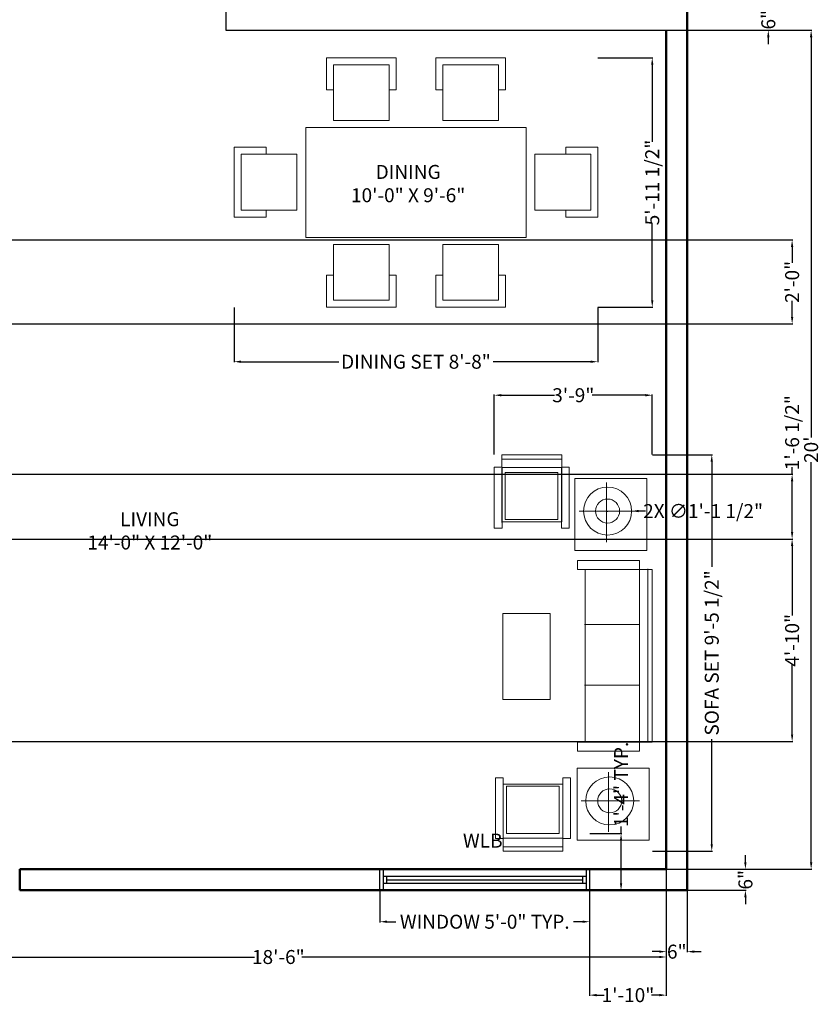
# Model space of a CAD drawing. Units: inches. Extents: x 2663 to 3147, y 140 to 736.
# Tile 3 of 6: x 2905 to 3134, y 144 to 425. Entities that reach past the tile are written whole.
import ezdxf

# ---------------------------------------------------------------- set-up
doc = ezdxf.new("R2010")
doc.units = ezdxf.units.IN
doc.header["$MEASUREMENT"] = 0
for name, color, linetype, lineweight in [('A-ANNO-DIMS', 2, 'Continuous', 18), ('A-AREA-IDEN', 3, 'Continuous', 25), ('A-FLOR-STRS', 1, 'Continuous', 25), ('A-FURN', 8, 'Continuous', 18), ('A-GLAZ', 4, 'Continuous', 25), ('A-WALL', 7, 'Continuous', 50)]:
    doc.layers.add(name, color=color, linetype=linetype, lineweight=lineweight)
doc.styles.get("Standard").update_dxf_attribs({"font": 'arial.ttf'})
doc.dimstyles.get("Standard").update_dxf_attribs({"dimtxt": 4, "dimasz": 2, "dimexe": 0.18, "dimexo": 0.0625, "dimgap": 0.09, "dimtad": 0, "dimdec": 0, "dimzin": 0, "dimdsep": 46, "dimlunit": 4, "dimtxsty": 'Standard', "dimcen": 0.09, "dimadec": 0, "dimazin": 0, "dimtfac": 1, "dimtdec": 0, "dimtofl": 0, "dimtmove": 0, "dimatfit": 3, "dimfxl": 1, "dimtolj": 1, "dimtzin": 0, "dimarcsym": 0})

# ---------------------------------------------------------------- blocks, each defined once
blk = doc.blocks.new('EDFRTYUI')
for p, q in [((3325.9, 253.54), (3325.9, 259.54)), ((3325.9, 259.54), (3385.9, 259.54)), ((3326.9, 253.54), (3326.9, 259.54)), ((3384.9, 259.54), (3384.9, 253.54)), ((3385.9, 259.54), (3385.9, 253.54)), ((3326.9, 257.54), (3384.9, 257.54)), ((3327.9, 255.54), (3327.9, 257.54)), ((3327.9, 256.54), (3383.9, 256.54)), ((3383.9, 257.54), (3383.9, 255.54)), ((3385.9, 253.54), (3325.9, 253.54)), ((3326.9, 255.54), (3384.9, 255.54))]:
    blk.add_line(p, q)
at = {"insert": (3337.87, 269.72), "char_height": 4, "attachment_point": 1}
blk.add_mtext_dynamic_manual_height_columns('\\pxqc;WLB', width=34.9199, gutter_width=20, heights=[0], dxfattribs=at)
blk = doc.blocks.new('A$C30E17696')
for p, q in [((0.6703, 1.8113), (1.177, 1.8113)), ((0.6703, 1.8113), (0.6703, 1.5785)), ((1.177, 1.8113), (1.177, 1.5785)), ((1.9712, 1.8113), (1.4645, 1.8113)), ((1.4645, 1.8113), (1.4645, 1.5785)), ((1.9712, 1.8113), (1.9712, 1.5785)), ((0.7209, 1.7606), (0.7209, 1.3552)), ((0.7209, 1.7606), (1.1263, 1.7606)), ((1.1263, 1.7606), (1.1263, 1.3552)), ((1.5151, 1.7606), (1.5151, 1.3552)), ((1.9205, 1.7606), (1.5151, 1.7606)), ((1.9205, 1.7606), (1.9205, 1.3552)), ((0.6703, 1.5785), (0.7209, 1.5785)), ((1.1263, 1.5785), (1.177, 1.5785)), ((1.5151, 1.5785), (1.4645, 1.5785)), ((1.9712, 1.5785), (1.9205, 1.5785)), ((0.5207, 1.3056), (0.5207, 0.5056)), ((2.1207, 1.3056), (0.5207, 1.3056)), ((0.7209, 1.3552), (1.1263, 1.3552)), ((1.9205, 1.3552), (1.5151, 1.3552)), ((2.1207, 0.5056), (2.1207, 1.3056)), ((0, 0.6545), (0, 1.1613)), ((0, 1.1613), (0.2327, 1.1613)), ((0.2327, 1.1106), (0.2327, 1.1613)), ((2.6414, 1.1613), (2.4087, 1.1613)), ((2.4087, 1.1106), (2.4087, 1.1613)), ((2.6414, 0.6545), (2.6414, 1.1613)), ((0.0507, 0.7052), (0.0507, 1.1106)), ((0.0507, 1.1106), (0.456, 1.1106)), ((0.456, 0.7052), (0.456, 1.1106)), ((2.1854, 0.7052), (2.1854, 1.1106)), ((2.5907, 1.1106), (2.1854, 1.1106)), ((2.5907, 0.7052), (2.5907, 1.1106)), ((0, 0.6545), (0.2327, 0.6545)), ((0.0507, 0.7052), (0.456, 0.7052)), ((0.2327, 0.6545), (0.2327, 0.7052)), ((2.5907, 0.7052), (2.1854, 0.7052)), ((2.4087, 0.6545), (2.4087, 0.7052)), ((2.6414, 0.6545), (2.4087, 0.6545)), ((0.5207, 0.5056), (2.1207, 0.5056)), ((0.7209, 0.456), (1.1263, 0.456)), ((0.7209, 0.0507), (0.7209, 0.456)), ((1.1263, 0.0507), (1.1263, 0.456)), ((1.5151, 0.0507), (1.5151, 0.456)), ((1.9205, 0.456), (1.5151, 0.456)), ((1.9205, 0.0507), (1.9205, 0.456)), ((0.6703, 0), (0.6703, 0.2327)), ((0.6703, 0.2327), (0.7209, 0.2327)), ((1.1263, 0.2327), (1.177, 0.2327)), ((1.177, 0), (1.177, 0.2327)), ((1.4645, 0), (1.4645, 0.2327)), ((1.5151, 0.2327), (1.4645, 0.2327)), ((1.9712, 0.2327), (1.9205, 0.2327)), ((1.9712, 0), (1.9712, 0.2327)), ((0.7209, 0.0507), (1.1263, 0.0507)), ((1.9205, 0.0507), (1.5151, 0.0507)), ((0.6703, 0), (1.177, 0)), ((1.9712, 0), (1.4645, 0))]:
    blk.add_line(p, q)
blk = doc.blocks.new('A$C482A143B')
for p, q in [((952.8, 1281.2), (2397.2, 1281.2)), ((469.8, 1193.5), (469.8, 706.9)), ((952.8, 1210.8), (2397.2, 1210.8)), ((1416.2, 1204.9), (1416.2, 753.5)), ((1920.6, 1204.9), (1920.6, 753.5)), ((2886.7, 1211), (2886.7, 724.4)), ((231.4, 934.7), (729, 934.7)), ((2648.3, 952.2), (3145.8, 952.2)), ((36.9, 62), (36.9, 562)), ((107.2, 62), (107.2, 562)), ((3198.7, 72.9), (3198.7, 573)), ((3269.1, 72.9), (3269.1, 573)), ((107.2, 62), (0, 62)), ((113.1, 62), (564.6, 62)), ((3192.9, 72.9), (2741.4, 72.9)), ((3198.7, 72.9), (3305.9, 72.9))]:
    blk.add_line(p, q)
for points in [[(957.2, 758), (957.2, 1318), (2397.2, 1318), (2397.2, 758)], [(797.5, 672.9), (197.5, 672.9), (197.5, 1272.9), (797.5, 1272.9)], [(3214.3, 690.4), (2614.3, 690.4), (2614.3, 1290.4), (3214.3, 1290.4)], [(883, 694), (883, 1210.8), (957.2, 1210.8), (957.2, 694)], [(2471.3, 694), (2471.3, 1210.8), (2397.2, 1210.8), (2397.2, 694)], [(611.7, 559.6), (105.3, 559.6), (105.3, 624), (611.7, 624)], [(2694.3, 570.6), (3200.7, 570.6), (3200.7, 634.9), (2694.3, 634.9)], [(541.1, 91.3), (148.3, 91.3), (148.3, 531.2), (541.1, 531.2)], [(2764.8, 102.3), (3157.7, 102.3), (3157.7, 542.2), (2764.8, 542.2)], [(1325.3, 466.6), (2040.7, 466.6), (2040.7, 72.4), (1325.3, 72.4)], [(611.7, 64.4), (105.3, 64.4), (105.3, 0), (611.7, 0)], [(2694.3, 75.4), (3200.7, 75.4), (3200.7, 11), (2694.3, 11)]]:
    blk.add_lwpolyline(points, close=True)
for points in [[(0, 62), (0, 562), (560, 562), (560, 62)], [(3305.9, 72.9), (3305.9, 573), (2745.9, 573), (2745.9, 72.9)]]:
    blk.add_lwpolyline(points)
for centre, radius in [((2886.7, 962.5), 200), ((469.8, 945), 200), ((469.8, 945), 100), ((2886.7, 962.5), 100)]:
    blk.add_circle(centre, radius)
at = {"width": 0.8, "flags": 9}
for tag in ['XSIZE', 'YSIZE']:
    blk.add_attdef(tag, (1677.2, 758), '', height=0.4, dxfattribs=at)
for tag in ['XSIZE', 'YSIZE']:
    blk.add_attdef(tag, (541.1, 311.2), '', height=0.4, rotation=90, dxfattribs=at)
at = {"text_generation_flag": 2, "width": 0.8, "flags": 9}
for tag in ['YSIZE', 'XSIZE']:
    blk.add_attdef(tag, (2764.8, 322.2), '', height=0.4, rotation=270, dxfattribs=at)
blk = doc.blocks.new('*D25')
at = {"layer": 'A-ANNO-DIMS', "color": 0, "lineweight": -2, "transparency": 16777216}
for p, q in [((3119.35, 430.32), (3119.35, 432.32)), ((3096.22, 428.32), (3119.53, 428.32)), ((3096.22, 422.32), (3119.53, 422.32)), ((3119.35, 420.32), (3119.35, 418.32))]:
    blk.add_line(p, q, dxfattribs=at)
at = {"layer": 'A-ANNO-DIMS', "color": 0, "transparency": 16777216}
for points in [[(3119.01, 430.32), (3119.68, 430.32), (3119.35, 428.32)], [(3119.01, 420.32), (3119.68, 420.32), (3119.35, 422.32)]]:
    blk.add_solid(points, dxfattribs=at)
at = {"layer": 'Defpoints', "color": 0, "transparency": 16777216}
for p in [(3096.16, 428.32), (3096.16, 422.32), (3119.35, 422.32)]:
    blk.add_point(p, dxfattribs=at)
at = {"layer": 'A-ANNO-DIMS', "color": 0, "transparency": 16777216, "insert": (3119.35, 425.32), "char_height": 4, "attachment_point": 5, "rotation": 90}
blk.add_mtext('\\A1;6"', dxfattribs=at)
blk = doc.blocks.new('*D26')
at = {"layer": 'A-ANNO-DIMS', "color": 0, "lineweight": -2, "transparency": 16777216}
for p, q in [((3090.22, 422.32), (3131.78, 422.32)), ((3131.6, 420.32), (3131.6, 305.84)), ((3131.6, 184.32), (3131.6, 298.81)), ((3090.22, 182.32), (3131.78, 182.32))]:
    blk.add_line(p, q, dxfattribs=at)
at = {"layer": 'A-ANNO-DIMS', "color": 0, "transparency": 16777216}
for points in [[(3131.27, 420.32), (3131.94, 420.32), (3131.6, 422.32)], [(3131.27, 184.32), (3131.94, 184.32), (3131.6, 182.32)]]:
    blk.add_solid(points, dxfattribs=at)
at = {"layer": 'Defpoints', "color": 0, "transparency": 16777216}
for p in [(3090.16, 422.32), (3090.16, 182.32), (3131.6, 182.32)]:
    blk.add_point(p, dxfattribs=at)
at = {"layer": 'A-ANNO-DIMS', "color": 0, "transparency": 16777216, "insert": (3131.6, 302.32), "char_height": 4, "attachment_point": 5, "rotation": 90}
blk.add_mtext("\\A1;20'", dxfattribs=at)
blk = doc.blocks.new('*D27')
at = {"layer": 'A-ANNO-DIMS', "color": 0, "lineweight": -2, "transparency": 16777216}
for p, q in [((2868.16, 182.26), (2868.16, 157.05)), ((3090.16, 182.26), (3090.16, 157.05)), ((2870.16, 157.23), (2972.39, 157.23)), ((3088.16, 157.23), (2985.93, 157.23))]:
    blk.add_line(p, q, dxfattribs=at)
at = {"layer": 'A-ANNO-DIMS', "color": 0, "transparency": 16777216}
for points in [[(2870.16, 157.56), (2870.16, 156.89), (2868.16, 157.23)], [(3088.16, 157.56), (3088.16, 156.89), (3090.16, 157.23)]]:
    blk.add_solid(points, dxfattribs=at)
at = {"layer": 'Defpoints', "color": 0, "transparency": 16777216}
for p in [(2868.16, 182.32), (3090.16, 182.32), (2868.16, 157.23)]:
    blk.add_point(p, dxfattribs=at)
at = {"layer": 'A-ANNO-DIMS', "color": 0, "transparency": 16777216, "insert": (2979.16, 157.23), "char_height": 4, "attachment_point": 5}
blk.add_mtext('\\A1;18\'-6"', dxfattribs=at)
blk = doc.blocks.new('*D28')
at = {"layer": 'A-ANNO-DIMS', "color": 0, "lineweight": -2, "transparency": 16777216}
for p, q in [((3090.16, 182.26), (3090.16, 158.58)), ((3096.16, 176.26), (3096.16, 158.58)), ((3088.16, 158.76), (3086.16, 158.76)), ((3098.16, 158.76), (3100.16, 158.76))]:
    blk.add_line(p, q, dxfattribs=at)
at = {"layer": 'A-ANNO-DIMS', "color": 0, "transparency": 16777216}
for points in [[(3088.16, 159.1), (3088.16, 158.43), (3090.16, 158.76)], [(3098.16, 159.1), (3098.16, 158.43), (3096.16, 158.76)]]:
    blk.add_solid(points, dxfattribs=at)
at = {"layer": 'Defpoints', "color": 0, "transparency": 16777216}
for p in [(3090.16, 182.32), (3096.16, 176.32), (3090.16, 158.76)]:
    blk.add_point(p, dxfattribs=at)
at = {"layer": 'A-ANNO-DIMS', "color": 0, "transparency": 16777216, "insert": (3093.16, 158.76), "char_height": 4, "attachment_point": 5}
blk.add_mtext('\\A1;6"', dxfattribs=at)
blk = doc.blocks.new('*D29')
at = {"layer": 'A-ANNO-DIMS', "color": 0, "lineweight": -2, "transparency": 16777216}
for p, q in [((3112.8, 184.32), (3112.8, 186.32)), ((3090.22, 182.32), (3112.98, 182.32)), ((3096.22, 176.32), (3112.98, 176.32)), ((3112.8, 174.32), (3112.8, 172.32))]:
    blk.add_line(p, q, dxfattribs=at)
at = {"layer": 'A-ANNO-DIMS', "color": 0, "transparency": 16777216}
for points in [[(3112.46, 184.32), (3113.13, 184.32), (3112.8, 182.32)], [(3112.46, 174.32), (3113.13, 174.32), (3112.8, 176.32)]]:
    blk.add_solid(points, dxfattribs=at)
at = {"layer": 'Defpoints', "color": 0, "transparency": 16777216}
for p in [(3090.16, 182.32), (3112.8, 182.32), (3096.16, 176.32)]:
    blk.add_point(p, dxfattribs=at)
at = {"layer": 'A-ANNO-DIMS', "color": 0, "transparency": 16777216, "insert": (3112.8, 179.32), "char_height": 4, "attachment_point": 5, "rotation": 90}
blk.add_mtext('\\A1;6"', dxfattribs=at)
blk = doc.blocks.new('*D41')
at = {"layer": 'A-ANNO-DIMS', "color": 0, "lineweight": -2, "transparency": 16777216}
for p, q in [((3008.22, 176.26), (3008.22, 167.14)), ((3068.22, 176.26), (3068.22, 167.14)), ((3010.22, 167.32), (3012.82, 167.32)), ((3066.22, 167.32), (3063.62, 167.32))]:
    blk.add_line(p, q, dxfattribs=at)
at = {"layer": 'A-ANNO-DIMS', "color": 0, "transparency": 16777216}
for points in [[(3010.22, 167.66), (3010.22, 166.99), (3008.22, 167.32)], [(3066.22, 167.66), (3066.22, 166.99), (3068.22, 167.32)]]:
    blk.add_solid(points, dxfattribs=at)
at = {"layer": 'Defpoints', "color": 0, "transparency": 16777216}
for p in [(3008.22, 176.32), (3068.22, 176.32), (3068.22, 167.32)]:
    blk.add_point(p, dxfattribs=at)
at = {"layer": 'A-ANNO-DIMS', "color": 0, "transparency": 16777216, "insert": (3038.22, 167.32), "char_height": 4, "attachment_point": 5}
blk.add_mtext('\\A1;WINDOW 5\'-0" TYP.', dxfattribs=at)
blk = doc.blocks.new('*D42')
at = {"layer": 'A-ANNO-DIMS', "color": 0, "lineweight": -2, "transparency": 16777216}
for p, q in [((3077.22, 192.51), (3077.22, 194.51)), ((3068.28, 192.51), (3077.4, 192.51)), ((3077.22, 178.32), (3077.22, 190.51)), ((3068.28, 176.32), (3077.4, 176.32))]:
    blk.add_line(p, q, dxfattribs=at)
at = {"layer": 'A-ANNO-DIMS', "color": 0, "transparency": 16777216}
for points in [[(3076.89, 190.51), (3077.55, 190.51), (3077.22, 192.51)], [(3076.89, 178.32), (3077.55, 178.32), (3077.22, 176.32)]]:
    blk.add_solid(points, dxfattribs=at)
at = {"layer": 'Defpoints', "color": 0, "transparency": 16777216}
for p in [(3068.22, 192.51), (3077.22, 192.51), (3068.22, 176.32)]:
    blk.add_point(p, dxfattribs=at)
at = {"layer": 'A-ANNO-DIMS', "color": 0, "transparency": 16777216, "insert": (3077.22, 206.6), "char_height": 4, "attachment_point": 5, "rotation": 90}
blk.add_mtext('\\A1;1\'-4" TYP.', dxfattribs=at)
blk = doc.blocks.new('*D57')
at = {"layer": 'A-ANNO-DIMS', "color": 0, "lineweight": -2, "transparency": 16777216}
for p, q in [((2966.52, 343.04), (2966.52, 327.32)), ((3070.54, 343.04), (3070.54, 327.32)), ((2968.52, 327.5), (2996.46, 327.5)), ((3068.54, 327.5), (3040.6, 327.5))]:
    blk.add_line(p, q, dxfattribs=at)
at = {"layer": 'A-ANNO-DIMS', "color": 0, "transparency": 16777216}
for points in [[(2968.52, 327.83), (2968.52, 327.16), (2966.52, 327.5)], [(3068.54, 327.83), (3068.54, 327.16), (3070.54, 327.5)]]:
    blk.add_solid(points, dxfattribs=at)
at = {"layer": 'Defpoints', "color": 0, "transparency": 16777216}
for p in [(2966.52, 343.1), (3070.54, 343.1), (3070.54, 327.5)]:
    blk.add_point(p, dxfattribs=at)
at = {"layer": 'A-ANNO-DIMS', "color": 0, "transparency": 16777216, "insert": (3018.53, 327.5), "char_height": 4, "attachment_point": 5}
blk.add_mtext('\\A1;DINING SET 8\'-8"', dxfattribs=at)
blk = doc.blocks.new('*D58')
at = {"layer": 'A-ANNO-DIMS', "color": 0, "lineweight": -2, "transparency": 16777216}
for p, q in [((3070.6, 414.42), (3086.32, 414.42)), ((3086.14, 412.42), (3086.14, 390.38)), ((3086.14, 345.1), (3086.14, 367.14)), ((3070.6, 343.1), (3086.32, 343.1))]:
    blk.add_line(p, q, dxfattribs=at)
at = {"layer": 'A-ANNO-DIMS', "color": 0, "transparency": 16777216}
for points in [[(3085.81, 412.42), (3086.47, 412.42), (3086.14, 414.42)], [(3085.81, 345.1), (3086.47, 345.1), (3086.14, 343.1)]]:
    blk.add_solid(points, dxfattribs=at)
at = {"layer": 'Defpoints', "color": 0, "transparency": 16777216}
for p in [(3070.54, 414.42), (3086.14, 414.42), (3070.54, 343.1)]:
    blk.add_point(p, dxfattribs=at)
at = {"layer": 'A-ANNO-DIMS', "color": 0, "transparency": 16777216, "insert": (3086.14, 378.76), "char_height": 4, "attachment_point": 5, "rotation": 90}
blk.add_mtext('\\A1;5\'-11 1/2"', dxfattribs=at)
blk = doc.blocks.new('*D59')
at = {"layer": 'A-ANNO-DIMS', "color": 0, "lineweight": -2, "transparency": 16777216}
for p, q in [((3086.22, 300.9), (3103.35, 300.9)), ((3103.17, 298.9), (3103.17, 268.85)), ((3103.17, 189.49), (3103.17, 219.54)), ((3086.22, 187.49), (3103.35, 187.49))]:
    blk.add_line(p, q, dxfattribs=at)
at = {"layer": 'A-ANNO-DIMS', "color": 0, "transparency": 16777216}
for points in [[(3102.84, 298.9), (3103.5, 298.9), (3103.17, 300.9)], [(3102.84, 189.49), (3103.5, 189.49), (3103.17, 187.49)]]:
    blk.add_solid(points, dxfattribs=at)
at = {"layer": 'Defpoints', "color": 0, "transparency": 16777216}
for p in [(3086.16, 300.9), (3086.16, 187.49), (3103.17, 187.49)]:
    blk.add_point(p, dxfattribs=at)
at = {"layer": 'A-ANNO-DIMS', "color": 0, "transparency": 16777216, "insert": (3103.17, 244.2), "char_height": 4, "attachment_point": 5, "rotation": 90}
blk.add_mtext('\\A1;SOFA SET 9\'-5 1/2"', dxfattribs=at)
blk = doc.blocks.new('*D60')
at = {"layer": 'A-ANNO-DIMS', "color": 0, "lineweight": -2, "transparency": 16777216}
for p, q in [((3040.95, 300.96), (3040.95, 318.09)), ((3042.95, 317.91), (3058.15, 317.91)), ((3084.16, 317.91), (3068.96, 317.91)), ((3086.16, 300.96), (3086.16, 318.09))]:
    blk.add_line(p, q, dxfattribs=at)
at = {"layer": 'A-ANNO-DIMS', "color": 0, "transparency": 16777216}
for points in [[(3042.95, 318.24), (3042.95, 317.58), (3040.95, 317.91)], [(3084.16, 318.24), (3084.16, 317.58), (3086.16, 317.91)]]:
    blk.add_solid(points, dxfattribs=at)
at = {"layer": 'Defpoints', "color": 0, "transparency": 16777216}
for p in [(3086.16, 317.91), (3040.95, 300.9), (3086.16, 300.9)]:
    blk.add_point(p, dxfattribs=at)
at = {"layer": 'A-ANNO-DIMS', "color": 0, "transparency": 16777216, "insert": (3063.55, 317.91), "char_height": 4, "attachment_point": 5}
blk.add_mtext('\\A1;3\'-9"', dxfattribs=at)
blk = doc.blocks.new('*D64')
at = {"layer": 'A-ANNO-DIMS', "color": 0, "lineweight": -2, "transparency": 16777216}
for p, q in [((2878.36, 276.78), (3126.34, 276.78)), ((3126.16, 274.78), (3126.16, 254.86)), ((3126.16, 220.86), (3126.16, 240.78)), ((2878.36, 218.86), (3126.34, 218.86))]:
    blk.add_line(p, q, dxfattribs=at)
at = {"layer": 'A-ANNO-DIMS', "color": 0, "transparency": 16777216}
for points in [[(3125.83, 274.78), (3126.49, 274.78), (3126.16, 276.78)], [(3125.83, 220.86), (3126.49, 220.86), (3126.16, 218.86)]]:
    blk.add_solid(points, dxfattribs=at)
at = {"layer": 'Defpoints', "color": 0, "transparency": 16777216}
for p in [(2878.3, 276.78), (3126.16, 276.78), (2878.3, 218.86)]:
    blk.add_point(p, dxfattribs=at)
at = {"layer": 'A-ANNO-DIMS', "color": 0, "transparency": 16777216, "insert": (3126.16, 247.82), "char_height": 4, "attachment_point": 5, "rotation": 90}
blk.add_mtext('\\A1;4\'-10"', dxfattribs=at)
blk = doc.blocks.new('*D65')
at = {"layer": 'A-ANNO-DIMS', "color": 0, "lineweight": -2, "transparency": 16777216}
for p, q in [((3126.16, 295.32), (3126.16, 297.32)), ((2868.22, 295.32), (3126.34, 295.32)), ((3126.16, 278.78), (3126.16, 293.32)), ((2878.36, 276.78), (3126.34, 276.78))]:
    blk.add_line(p, q, dxfattribs=at)
at = {"layer": 'A-ANNO-DIMS', "color": 0, "transparency": 16777216}
for points in [[(3125.83, 293.32), (3126.49, 293.32), (3126.16, 295.32)], [(3125.83, 278.78), (3126.49, 278.78), (3126.16, 276.78)]]:
    blk.add_solid(points, dxfattribs=at)
at = {"layer": 'Defpoints', "color": 0, "transparency": 16777216}
for p in [(2868.16, 295.32), (3126.16, 295.32), (2878.3, 276.78)]:
    blk.add_point(p, dxfattribs=at)
at = {"layer": 'A-ANNO-DIMS', "color": 0, "transparency": 16777216, "insert": (3126.16, 307.2), "char_height": 4, "attachment_point": 5, "rotation": 90}
blk.add_mtext('\\A1;1\'-6 1/2"', dxfattribs=at)
blk = doc.blocks.new('*D72')
at = {"layer": 'A-ANNO-DIMS', "color": 0, "lineweight": -2, "transparency": 16777216}
for p, q in [((3068.22, 182.26), (3068.22, 146.14)), ((3090.16, 182.26), (3090.16, 146.14)), ((3070.22, 146.32), (3072.42, 146.32)), ((3088.16, 146.32), (3085.96, 146.32))]:
    blk.add_line(p, q, dxfattribs=at)
at = {"layer": 'A-ANNO-DIMS', "color": 0, "transparency": 16777216}
for points in [[(3070.22, 146.66), (3070.22, 145.99), (3068.22, 146.32)], [(3088.16, 146.66), (3088.16, 145.99), (3090.16, 146.32)]]:
    blk.add_solid(points, dxfattribs=at)
at = {"layer": 'Defpoints', "color": 0, "transparency": 16777216}
for p in [(3068.22, 182.32), (3090.16, 182.32), (3090.16, 146.32)]:
    blk.add_point(p, dxfattribs=at)
at = {"layer": 'A-ANNO-DIMS', "color": 0, "transparency": 16777216, "insert": (3079.19, 146.32), "char_height": 4, "attachment_point": 5}
blk.add_mtext('\\A1;1\'-10"', dxfattribs=at)
blk = doc.blocks.new('*D84')
at = {"layer": 'A-ANNO-DIMS', "color": 0, "lineweight": -2, "transparency": 16777216}
for p, q in [((2809.05, 362.32), (3126.34, 362.32)), ((3126.16, 360.32), (3126.16, 355.76)), ((3126.16, 340.32), (3126.16, 344.88)), ((2809.05, 338.32), (3126.34, 338.32))]:
    blk.add_line(p, q, dxfattribs=at)
at = {"layer": 'A-ANNO-DIMS', "color": 0, "transparency": 16777216}
for points in [[(3125.83, 360.32), (3126.49, 360.32), (3126.16, 362.32)], [(3125.83, 340.32), (3126.49, 340.32), (3126.16, 338.32)]]:
    blk.add_solid(points, dxfattribs=at)
at = {"layer": 'Defpoints', "color": 0, "transparency": 16777216}
for p in [(2808.99, 362.32), (3126.16, 362.32), (2808.99, 338.32)]:
    blk.add_point(p, dxfattribs=at)
at = {"layer": 'A-ANNO-DIMS', "color": 0, "transparency": 16777216, "insert": (3126.16, 350.32), "char_height": 4, "attachment_point": 5, "rotation": 90}
blk.add_mtext('\\A1;2\'-0"', dxfattribs=at)
blk = doc.blocks.new('*D89')
at = {"layer": 'A-ANNO-DIMS', "color": 0, "lineweight": -2, "transparency": 16777216}
for p, q in [((3073.27, 284.78), (3073.45, 284.78)), ((3073.36, 284.69), (3073.36, 284.87)), ((3084.22, 284.78), (3082.22, 284.78))]:
    blk.add_line(p, q, dxfattribs=at)
at = {"layer": 'A-ANNO-DIMS', "color": 0, "transparency": 16777216}
blk.add_solid([(3082.22, 285.11), (3082.22, 284.45), (3080.22, 284.78)], dxfattribs=at)
at = {"layer": 'Defpoints', "color": 0, "transparency": 16777216}
for p in [(3066.5, 284.78), (3080.22, 284.78)]:
    blk.add_point(p, dxfattribs=at)
at = {"layer": 'A-ANNO-DIMS', "color": 0, "transparency": 16777216, "insert": (3100.69, 284.78), "char_height": 4, "attachment_point": 5, "rotation": 0.0035}
blk.add_mtext('\\A1;2X ∅1\'-1 1/2"', dxfattribs=at)

msp = doc.modelspace()

# ---------------------------------------------------------------- linework, layer by layer
at = {"layer": 'A-FLOR-STRS'}
for p, q in [((2964.16, 462.32), (2964.16, 422.32)), ((2964.16, 422.32), (3090.16, 422.32))]:
    msp.add_line(p, q, dxfattribs=at)
at = {"layer": 'A-WALL'}
for p, q in [((3096.16, 656.32), (3096.16, 176.32)), ((3090.16, 422.32), (3090.16, 182.32)), ((3090.16, 182.32), (2905.16, 182.32)), ((2905.16, 176.32), (2905.16, 182.32)), ((3096.16, 176.32), (2905.16, 176.32))]:
    msp.add_line(p, q, dxfattribs=at)

# ---------------------------------------------------------------- block references
at = {"layer": 'A-FURN', "xscale": 39.3790407916365, "yscale": 39.3790407916365, "zscale": 39.3790407916365}
msp.add_blockref('A$C30E17696', (2966.52, 343.1), dxfattribs=at)
at = {"layer": 'A-FURN', "xscale": 0.0343036435144511, "yscale": 0.0343036435144511, "zscale": 0.0343036435144511, "rotation": 270}
msp.add_blockref('A$C482A143B', (3040.95, 300.9), dxfattribs=at)
at = {"layer": 'A-GLAZ'}
msp.add_blockref('EDFRTYUI', (-317.68, -77.21), dxfattribs=at)

# ---------------------------------------------------------------- texts
at = {"layer": 'A-AREA-IDEN', "char_height": 4, "attachment_point": 1}
for s, width, insert in [('\\pxqc;DINING\\P10\'-0" X 9\'-6"', 63.7224, (2984.44, 383.78)), ('\\pxqc;LIVING \\P14\'-0" X 12\'-0" ', 81.0452, (2901.88, 284.45))]:
    msp.add_mtext_dynamic_manual_height_columns(s, width=width, gutter_width=20, heights=[0], dxfattribs=dict(at, insert=insert))

# ---------------------------------------------------------------- dimensions: what is measured, and where the dimension line sits
at = {"layer": 'A-ANNO-DIMS'}
for base, p1, p2, override, picture, middle in [((3119.35, 422.32), (3096.16, 428.32), (3096.16, 422.32), {"dimclrd": 0, "dimclre": 0, "dimclrt": 0}, '*D25', (3119.35, 425.32)), ((3131.6, 182.32), (3090.16, 422.32), (3090.16, 182.32), {"dimclrd": 0, "dimclre": 0, "dimclrt": 0}, '*D26', (3131.6, 302.32)), ((3086.14, 414.42), (3070.54, 343.1), (3070.54, 414.42), {"dimdec": 1, "dimrnd": 0, "dimzin": 1, "dimlunit": 4, "dimfrac": 2}, '*D58', (3086.14, 378.76)), ((3126.16, 362.32), (2808.99, 338.32), (2808.99, 362.32), {"dimdec": 1, "dimlfac": 1, "dimrnd": 0, "dimzin": 1, "dimdsep": 46, "dimlunit": 4, "dimfrac": 2}, '*D84', (3126.16, 350.32)), ((3126.16, 295.32), (2878.3, 276.78), (2868.16, 295.32), {"dimdec": 1, "dimlfac": 1, "dimrnd": 0, "dimzin": 1, "dimdsep": 46, "dimlunit": 4, "dimfrac": 2}, '*D65', (3126.16, 307.2)), ((3126.16, 276.78), (2878.3, 218.86), (2878.3, 276.78), {"dimdec": 1, "dimlfac": 1, "dimrnd": 0, "dimzin": 1, "dimdsep": 46, "dimlunit": 4, "dimfrac": 2}, '*D64', (3126.16, 247.82)), ((3112.8, 182.32), (3096.16, 176.32), (3090.16, 182.32), {"dimclrd": 0, "dimclre": 0, "dimclrt": 0}, '*D29', (3112.8, 179.32))]:
    dim = msp.add_linear_dim(base=base, p1=p1, p2=p2, angle=90, dimstyle='Standard', override=override, dxfattribs=at)
    dim.commit()
    dim.dimension.update_dxf_attribs({"geometry": picture, "text_midpoint": middle})
for base, p1, p2, text, picture, middle in [((3070.54, 327.5), (2966.52, 343.1), (3070.54, 343.1), 'DINING SET <>', '*D57', (3018.53, 327.5)), ((3068.22, 167.32), (3008.22, 176.32), (3068.22, 176.32), 'WINDOW <> TYP.', '*D41', (3038.22, 167.32))]:
    dim = msp.add_linear_dim(base=base, p1=p1, p2=p2, text=text, dimstyle='Standard', override={"dimdec": 1, "dimrnd": 0, "dimzin": 1, "dimlunit": 4, "dimfrac": 2}, dxfattribs=at)
    dim.commit()
    dim.dimension.update_dxf_attribs({"geometry": picture, "text_midpoint": middle})
for base, p1, p2, override, picture, middle in [((3086.16, 317.91), (3040.95, 300.9), (3086.16, 300.9), {"dimdec": 1, "dimrnd": 0, "dimzin": 1, "dimlunit": 4, "dimfrac": 2}, '*D60', (3063.55, 317.91)), ((2868.16, 157.23), (3090.16, 182.32), (2868.16, 182.32), {"dimclrd": 0, "dimclre": 0, "dimclrt": 0}, '*D27', (2979.16, 157.23)), ((3090.16, 146.32), (3068.22, 182.32), (3090.16, 182.32), {"dimdec": 1, "dimlfac": 1, "dimrnd": 0, "dimzin": 1, "dimdsep": 46, "dimlunit": 4, "dimfrac": 2}, '*D72', (3079.19, 146.32)), ((3090.16, 158.76), (3096.16, 176.32), (3090.16, 182.32), {"dimclrd": 0, "dimclre": 0, "dimclrt": 0}, '*D28', (3093.16, 158.76))]:
    dim = msp.add_linear_dim(base=base, p1=p1, p2=p2, dimstyle='Standard', override=override, dxfattribs=at)
    dim.commit()
    dim.dimension.update_dxf_attribs({"geometry": picture, "text_midpoint": middle})
for base, p1, p2, angle, text, picture, middle in [((3103.17, 187.49), (3086.16, 300.9), (3086.16, 187.49), 270, 'SOFA SET <>', '*D59', (3103.17, 244.2)), ((3077.22, 192.51), (3068.22, 176.32), (3068.22, 192.51), 90, '<> TYP.', '*D42', (3077.22, 206.6))]:
    dim = msp.add_linear_dim(base=base, p1=p1, p2=p2, angle=angle, text=text, dimstyle='Standard', override={"dimdec": 1, "dimrnd": 0, "dimzin": 1, "dimlunit": 4, "dimfrac": 2}, dxfattribs=at)
    dim.commit()
    dim.dimension.update_dxf_attribs({"geometry": picture, "text_midpoint": middle})
dim = msp.add_diameter_dim_2p(p1=(3066.5, 284.78), p2=(3080.22, 284.78), text='2X <>', dimstyle='Standard', override={"dimdec": 1, "dimlfac": 1, "dimrnd": 0, "dimzin": 1, "dimdsep": 46, "dimlunit": 4, "dimfrac": 2}, dxfattribs=at)
dim.commit()
dim.dimension.update_dxf_attribs({"geometry": '*D89', "text_midpoint": (3100.69, 284.78), "dimtype": 163})

doc.saveas('drawing.dxf')
